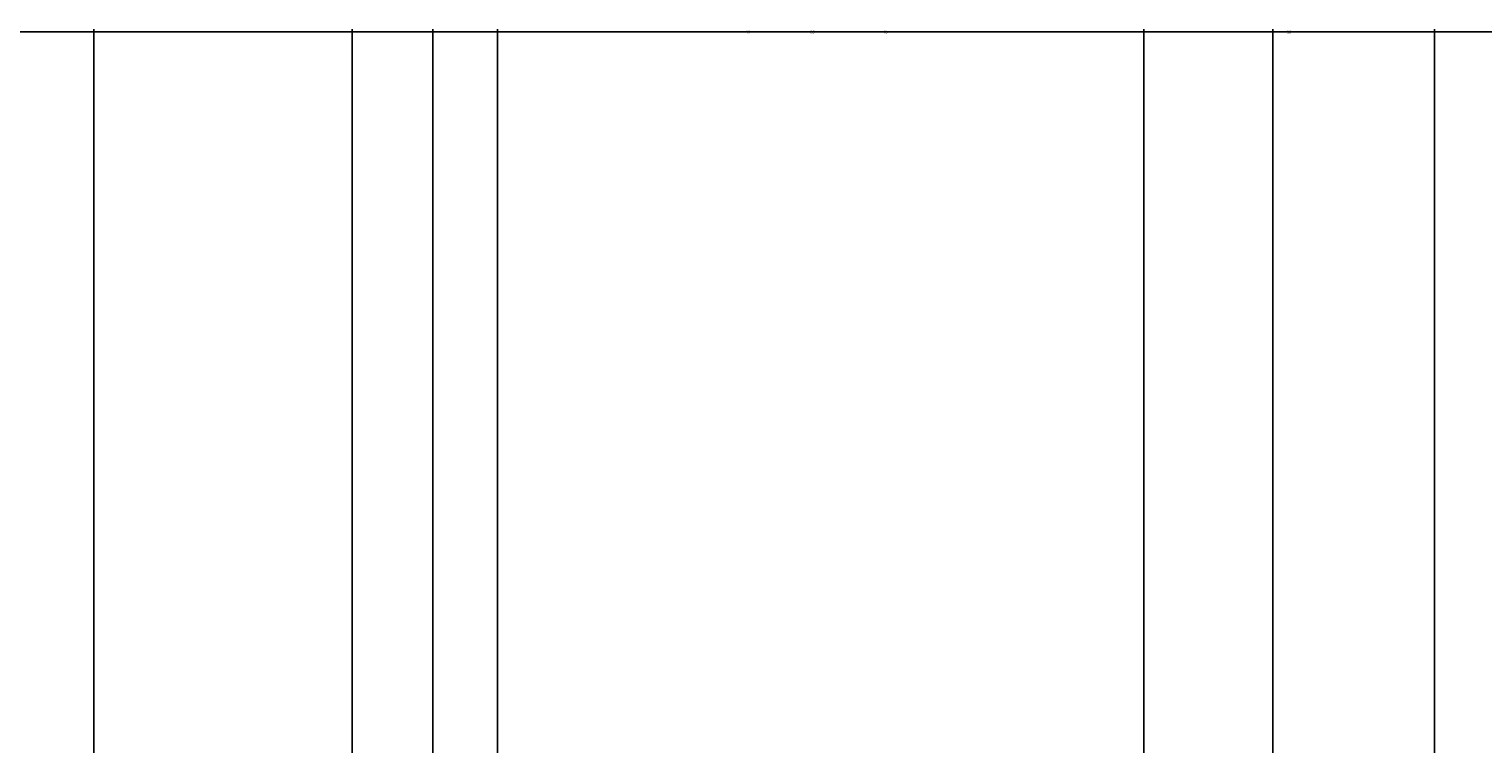
# Model space of a CAD drawing. Units: feet. Extents: x 105 to 1094, y -88 to 588.
# Tile 35 of 59: x 346 to 436, y 544 to 588. Entities that reach past the tile are written whole.
import ezdxf

# ---------------------------------------------------------------- set-up
doc = ezdxf.new("R2010")
doc.units = ezdxf.units.FT
doc.header["$MEASUREMENT"] = 0
doc.layers.add('A-ANNO-DIMS', color=2, linetype='Continuous', lineweight=18)
doc.styles.get("Standard").update_dxf_attribs({"font": 'arial.ttf'})
doc.dimstyles.get("Standard").update_dxf_attribs({"dimtxt": 0.18, "dimasz": 0.18, "dimexe": 0.18, "dimexo": 0.0625, "dimgap": 0.09, "dimtad": 0, "dimtih": 1, "dimtoh": 1, "dimdec": 4, "dimzin": 0, "dimdsep": 46, "dimtxsty": 'Standard', "dimcen": 0.09, "dimadec": 0, "dimazin": 0, "dimtfac": 1, "dimtdec": 4, "dimtofl": 0, "dimtmove": 0, "dimatfit": 3, "dimfxl": 1, "dimtolj": 1, "dimtzin": 0, "dimarcsym": 0})

# ---------------------------------------------------------------- blocks, each defined once
blk = doc.blocks.new('*D23')
at = {"layer": 'A-ANNO-DIMS', "color": 0, "lineweight": -2, "transparency": 16777216}
for p, q in [((231.688, 543.144), (231.688, 588.311)), ((231.868, 588.131), (290.408, 588.131)), ((349.508, 588.131), (290.969, 588.131)), ((349.688, 543.144), (349.688, 588.311))]:
    blk.add_line(p, q, dxfattribs=at)
at = {"layer": 'A-ANNO-DIMS', "color": 0, "transparency": 16777216}
for points in [[(231.868, 588.161), (231.868, 588.101), (231.688, 588.131)], [(349.508, 588.161), (349.508, 588.101), (349.688, 588.131)]]:
    blk.add_solid(points, dxfattribs=at)
at = {"layer": 'Defpoints', "color": 0, "transparency": 16777216}
for p in [(349.688, 588.131), (231.688, 543.081), (349.688, 543.081)]:
    blk.add_point(p, dxfattribs=at)
at = {"layer": 'A-ANNO-DIMS', "color": 0, "transparency": 16777216, "insert": (290.688, 588.131), "char_height": 0.18, "attachment_point": 5}
blk.add_mtext('\\A1;118', dxfattribs=at)
blk = doc.blocks.new('*D24')
at = {"layer": 'A-ANNO-DIMS', "color": 0, "lineweight": -2, "transparency": 16777216}
for p, q in [((349.688, 543.144), (349.688, 588.311)), ((349.868, 588.131), (393.969, 588.131)), ((438.508, 588.131), (394.408, 588.131)), ((438.688, 527.144), (438.688, 588.311))]:
    blk.add_line(p, q, dxfattribs=at)
at = {"layer": 'A-ANNO-DIMS', "color": 0, "transparency": 16777216}
for points in [[(349.868, 588.161), (349.868, 588.101), (349.688, 588.131)], [(438.508, 588.161), (438.508, 588.101), (438.688, 588.131)]]:
    blk.add_solid(points, dxfattribs=at)
at = {"layer": 'Defpoints', "color": 0, "transparency": 16777216}
for p in [(438.688, 588.131), (349.688, 543.081), (438.688, 527.081)]:
    blk.add_point(p, dxfattribs=at)
at = {"layer": 'A-ANNO-DIMS', "color": 0, "transparency": 16777216, "insert": (394.188, 588.131), "char_height": 0.18, "attachment_point": 5}
blk.add_mtext('\\A1;89', dxfattribs=at)
blk = doc.blocks.new('*D39')
at = {"layer": 'A-ANNO-DIMS', "color": 0, "lineweight": -2, "transparency": 16777216}
for p, q in [((294.688, 204.144), (294.688, 588.311)), ((294.868, 588.131), (332.47, 588.131)), ((370.508, 588.131), (332.906, 588.131)), ((370.688, 204.144), (370.688, 588.311))]:
    blk.add_line(p, q, dxfattribs=at)
at = {"layer": 'A-ANNO-DIMS', "color": 0, "transparency": 16777216}
for points in [[(294.868, 588.161), (294.868, 588.101), (294.688, 588.131)], [(370.508, 588.161), (370.508, 588.101), (370.688, 588.131)]]:
    blk.add_solid(points, dxfattribs=at)
at = {"layer": 'Defpoints', "color": 0, "transparency": 16777216}
for p in [(370.688, 588.131), (294.688, 204.081), (370.688, 204.081)]:
    blk.add_point(p, dxfattribs=at)
at = {"layer": 'A-ANNO-DIMS', "color": 0, "transparency": 16777216, "insert": (332.688, 588.131), "char_height": 0.18, "attachment_point": 5}
blk.add_mtext('\\A1;76', dxfattribs=at)
blk = doc.blocks.new('*D52')
at = {"layer": 'A-ANNO-DIMS', "color": 0, "lineweight": -2, "transparency": 16777216}
for p, q in [((414.688, 394.144), (414.688, 588.311)), ((414.868, 588.131), (423.478, 588.131)), ((432.508, 588.131), (423.899, 588.131)), ((432.688, 394.144), (432.688, 588.311))]:
    blk.add_line(p, q, dxfattribs=at)
at = {"layer": 'A-ANNO-DIMS', "color": 0, "transparency": 16777216}
for points in [[(414.868, 588.161), (414.868, 588.101), (414.688, 588.131)], [(432.508, 588.161), (432.508, 588.101), (432.688, 588.131)]]:
    blk.add_solid(points, dxfattribs=at)
at = {"layer": 'Defpoints', "color": 0, "transparency": 16777216}
for p in [(414.688, 588.131), (414.688, 394.081), (432.688, 394.081)]:
    blk.add_point(p, dxfattribs=at)
at = {"layer": 'A-ANNO-DIMS', "color": 0, "transparency": 16777216, "insert": (423.688, 588.131), "char_height": 0.18, "attachment_point": 5}
blk.add_mtext('\\A1;18', dxfattribs=at)
blk = doc.blocks.new('*D53')
at = {"layer": 'A-ANNO-DIMS', "color": 0, "lineweight": -2, "transparency": 16777216}
for p, q in [((365.688, 394.144), (365.688, 588.311)), ((365.868, 588.131), (389.966, 588.131)), ((414.508, 588.131), (390.411, 588.131)), ((414.688, 394.144), (414.688, 588.311))]:
    blk.add_line(p, q, dxfattribs=at)
at = {"layer": 'A-ANNO-DIMS', "color": 0, "transparency": 16777216}
for points in [[(365.868, 588.161), (365.868, 588.101), (365.688, 588.131)], [(414.508, 588.161), (414.508, 588.101), (414.688, 588.131)]]:
    blk.add_solid(points, dxfattribs=at)
at = {"layer": 'Defpoints', "color": 0, "transparency": 16777216}
for p in [(365.688, 588.131), (365.688, 394.081), (414.688, 394.081)]:
    blk.add_point(p, dxfattribs=at)
at = {"layer": 'A-ANNO-DIMS', "color": 0, "transparency": 16777216, "insert": (390.188, 588.131), "char_height": 0.18, "attachment_point": 5}
blk.add_mtext('\\A1;49', dxfattribs=at)
blk = doc.blocks.new('*D56')
at = {"layer": 'A-ANNO-DIMS', "color": 0, "lineweight": -2, "transparency": 16777216}
for p, q in [((374.688, 252.144), (374.688, 588.311)), ((374.868, 588.131), (398.466, 588.131)), ((422.508, 588.131), (398.911, 588.131)), ((422.688, 252.144), (422.688, 588.311))]:
    blk.add_line(p, q, dxfattribs=at)
at = {"layer": 'A-ANNO-DIMS', "color": 0, "transparency": 16777216}
for points in [[(374.868, 588.161), (374.868, 588.101), (374.688, 588.131)], [(422.508, 588.161), (422.508, 588.101), (422.688, 588.131)]]:
    blk.add_solid(points, dxfattribs=at)
at = {"layer": 'Defpoints', "color": 0, "transparency": 16777216}
for p in [(422.688, 588.131), (374.688, 252.081), (422.688, 252.081)]:
    blk.add_point(p, dxfattribs=at)
at = {"layer": 'A-ANNO-DIMS', "color": 0, "transparency": 16777216, "insert": (398.688, 588.131), "char_height": 0.18, "attachment_point": 5}
blk.add_mtext('\\A1;48', dxfattribs=at)

msp = doc.modelspace()

# ---------------------------------------------------------------- dimensions: what is measured, and where the dimension line sits
at = {"layer": 'A-ANNO-DIMS'}
for base, p1, p2, picture, middle in [((349.6883, 588.1312), (231.6883, 543.0812), (349.6883, 543.0812), '*D23', (290.6883, 588.1312)), ((370.6883, 588.1312), (294.6883, 204.0812), (370.6883, 204.0812), '*D39', (332.6883, 588.1312)), ((438.6883, 588.1312), (349.6883, 543.0812), (438.6883, 527.0812), '*D24', (394.1883, 588.1312)), ((365.6883, 588.1312), (414.6883, 394.0812), (365.6883, 394.0812), '*D53', (390.1883, 588.1312)), ((422.6883, 588.1312), (374.6883, 252.0812), (422.6883, 252.0812), '*D56', (398.6883, 588.1312)), ((414.6883, 588.1312), (432.6883, 394.0812), (414.6883, 394.0812), '*D52', (423.6883, 588.1312))]:
    dim = msp.add_linear_dim(base=base, p1=p1, p2=p2, dimstyle='Standard', override={"dimdec": 0, "dimlfac": 1, "dimrnd": 0, "dimzin": 0, "dimdsep": 46, "dimlunit": 2}, dxfattribs=at)
    dim.commit()
    dim.dimension.update_dxf_attribs({"geometry": picture, "text_midpoint": middle})

doc.saveas('drawing.dxf')
